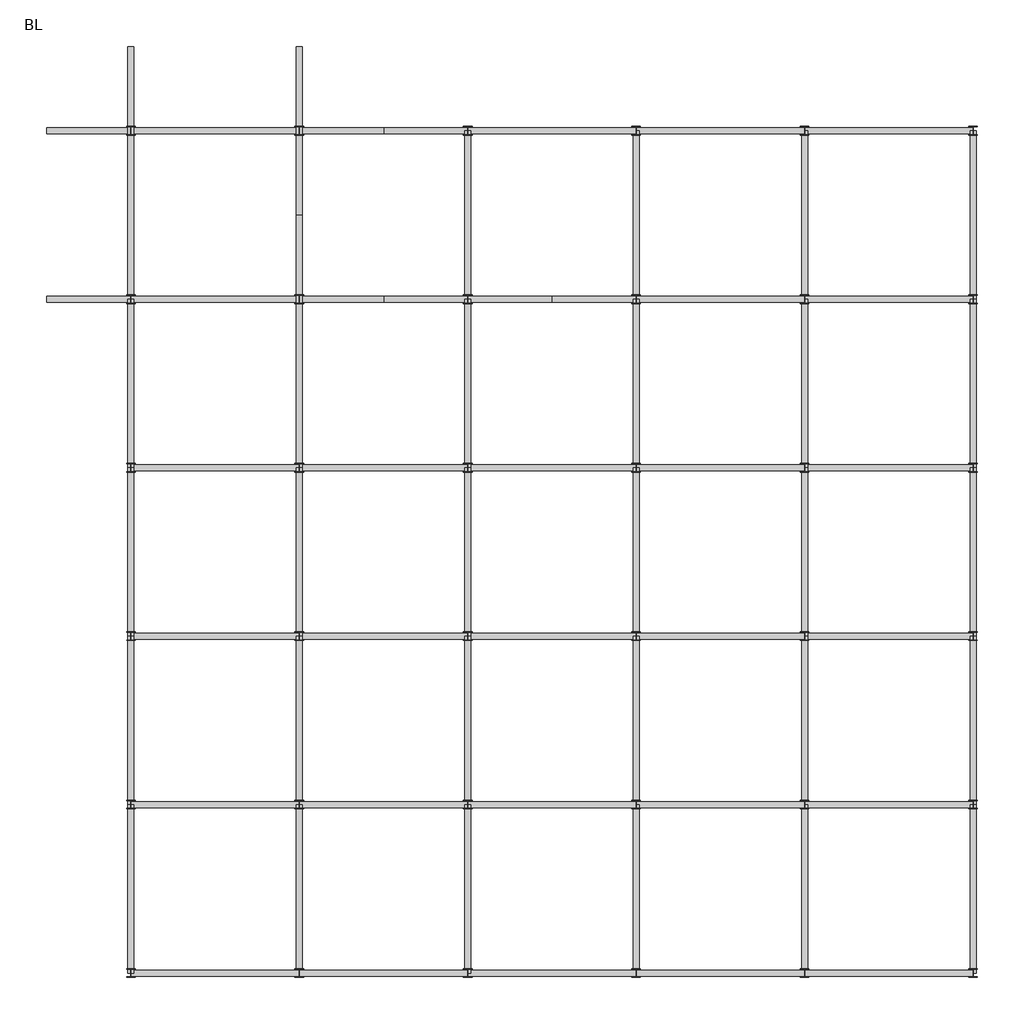
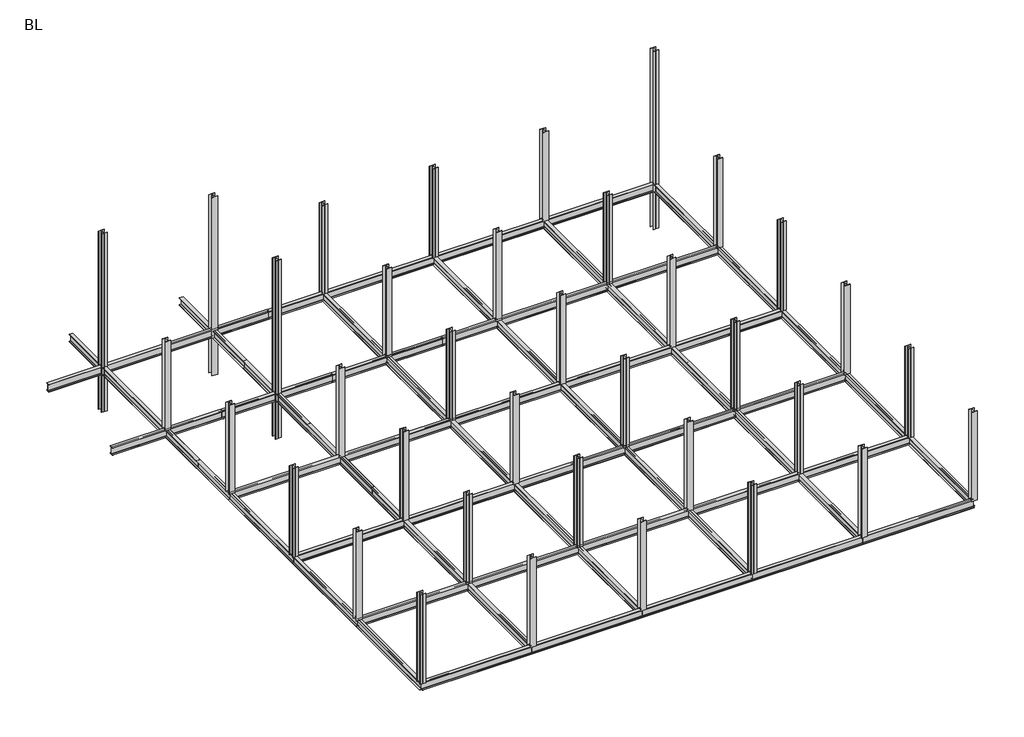
# One storey: 60 beams, 36 columns.
"""IFC4 building model written with IfcOpenShell, lengths in millimetres."""

from ifc_helpers import new_model, si_unit, origin, place, context, project, spatial, transform, mapped, element, save
from components import w_shapes_w14x30_541e514d, w_shapes_w14x30_920474df, w_shapes_column_w10x49_6b2d3d6a, w_shapes_column_w10x49_b9b2aca3

model = new_model("IFC4")

# Units and contexts
model_context = context("Model", 3, world=origin())
ifc_project = project(units=[si_unit("LENGTHUNIT", "METRE", prefix="MILLI")], contexts=[model_context])

# Site, building, storey
site = spatial("IfcSite", under=ifc_project)
building = spatial("IfcBuilding", under=site)
storey = spatial("IfcBuildingStorey", under=building, Name="BL", Elevation=4267.0)

# Beams
placement = place(None, origin())
w_shapes_w14x30_shape = w_shapes_w14x30_541e514d(model_context)
element("IfcBeam", 1, ObjectType="W Shapes : W14X30", at=placement, inside=storey, context=model_context, shape_type="MappedRepresentation", body=[
    mapped(w_shapes_w14x30_shape, transform((-15925.6378857, 14038.8625479, 4091.74), x_axis=(1.0, 0.0, 0.0), y_axis=(0.0, 1.0, 0.0), z_axis=(0.0, 0.0, 1.0))),
])
element("IfcBeam", 2, ObjectType="W Shapes : W14X30", at=placement, inside=storey, context=model_context, shape_type="MappedRepresentation", body=[
    mapped(w_shapes_w14x30_shape, transform((-15925.6378857, 19038.8625479, 4091.74), x_axis=(1.0, 0.0, 0.0), y_axis=(0.0, 1.0, 0.0), z_axis=(0.0, 0.0, 1.0))),
])
element("IfcBeam", 3, ObjectType="W Shapes : W14X30", at=placement, inside=storey, context=model_context, shape_type="MappedRepresentation", body=[
    mapped(w_shapes_w14x30_shape, transform((-13425.6378857, 11538.8625479, 4091.74), x_axis=(0.0, 1.0, 0.0), y_axis=(-1.0, 0.0, 0.0), z_axis=(0.0, 0.0, 1.0))),
])
element("IfcBeam", 4, ObjectType="W Shapes : W14X30", at=placement, inside=storey, context=model_context, shape_type="MappedRepresentation", body=[
    mapped(w_shapes_w14x30_shape, transform((-13425.6378857, 16538.8625479, 4091.74), x_axis=(0.0, 1.0, 0.0), y_axis=(-1.0, 0.0, 0.0), z_axis=(0.0, 0.0, 1.0))),
])
element("IfcBeam", 5, ObjectType="W Shapes : W14X30", at=placement, inside=storey, context=model_context, shape_type="MappedRepresentation", body=[
    mapped(w_shapes_w14x30_shape, transform((-18425.6378857, 16538.8625479, 4091.74), x_axis=(0.0, 1.0, 0.0), y_axis=(-1.0, 0.0, 0.0), z_axis=(0.0, 0.0, 1.0))),
])
element("IfcBeam", 6, ObjectType="W Shapes : W14X30", at=placement, inside=storey, context=model_context, shape_type="MappedRepresentation", body=[
    mapped(w_shapes_w14x30_shape, transform((-10925.6378857, 14038.8625479, 4091.74), x_axis=(1.0, 0.0, 0.0), y_axis=(0.0, 1.0, 0.0), z_axis=(0.0, 0.0, 1.0))),
])
w_shapes_w14x30_2_shape = w_shapes_w14x30_920474df(model_context)
element("IfcBeam", 7, ObjectType="W Shapes : W14X30", at=placement, inside=storey, context=model_context, shape_type="MappedRepresentation", body=[
    mapped(w_shapes_w14x30_2_shape, transform((-15925.6378857, -5961.1374521, 4091.74), x_axis=(1.0, 0.0, 0.0), y_axis=(0.0, 1.0, 0.0), z_axis=(0.0, 0.0, 1.0))),
])
element("IfcBeam", 8, ObjectType="W Shapes : W14X30", at=placement, inside=storey, context=model_context, shape_type="MappedRepresentation", body=[
    mapped(w_shapes_w14x30_2_shape, transform((-10925.6378857, -5961.1374521, 4091.74), x_axis=(1.0, 0.0, 0.0), y_axis=(0.0, 1.0, 0.0), z_axis=(0.0, 0.0, 1.0))),
])
element("IfcBeam", 9, ObjectType="W Shapes : W14X30", at=placement, inside=storey, context=model_context, shape_type="MappedRepresentation", body=[
    mapped(w_shapes_w14x30_2_shape, transform((-5925.6378857, -5961.1374521, 4091.74), x_axis=(1.0, 0.0, 0.0), y_axis=(0.0, 1.0, 0.0), z_axis=(0.0, 0.0, 1.0))),
])
element("IfcBeam", 10, ObjectType="W Shapes : W14X30", at=placement, inside=storey, context=model_context, shape_type="MappedRepresentation", body=[
    mapped(w_shapes_w14x30_2_shape, transform((-925.6378857, -5961.1374521, 4091.74), x_axis=(1.0, 0.0, 0.0), y_axis=(0.0, 1.0, 0.0), z_axis=(0.0, 0.0, 1.0))),
])
element("IfcBeam", 11, ObjectType="W Shapes : W14X30", at=placement, inside=storey, context=model_context, shape_type="MappedRepresentation", body=[
    mapped(w_shapes_w14x30_2_shape, transform((4074.3621143, -5961.1374521, 4091.74), x_axis=(1.0, 0.0, 0.0), y_axis=(0.0, 1.0, 0.0), z_axis=(0.0, 0.0, 1.0))),
])
element("IfcBeam", 12, ObjectType="W Shapes : W14X30", at=placement, inside=storey, context=model_context, shape_type="MappedRepresentation", body=[
    mapped(w_shapes_w14x30_2_shape, transform((-15925.6378857, -961.1374521, 4091.74), x_axis=(1.0, 0.0, 0.0), y_axis=(0.0, 1.0, 0.0), z_axis=(0.0, 0.0, 1.0))),
])
element("IfcBeam", 13, ObjectType="W Shapes : W14X30", at=placement, inside=storey, context=model_context, shape_type="MappedRepresentation", body=[
    mapped(w_shapes_w14x30_2_shape, transform((-10925.6378857, -961.1374521, 4091.74), x_axis=(1.0, 0.0, 0.0), y_axis=(0.0, 1.0, 0.0), z_axis=(0.0, 0.0, 1.0))),
])
element("IfcBeam", 14, ObjectType="W Shapes : W14X30", at=placement, inside=storey, context=model_context, shape_type="MappedRepresentation", body=[
    mapped(w_shapes_w14x30_2_shape, transform((-5925.6378857, -961.1374521, 4091.74), x_axis=(1.0, 0.0, 0.0), y_axis=(0.0, 1.0, 0.0), z_axis=(0.0, 0.0, 1.0))),
])
element("IfcBeam", 15, ObjectType="W Shapes : W14X30", at=placement, inside=storey, context=model_context, shape_type="MappedRepresentation", body=[
    mapped(w_shapes_w14x30_2_shape, transform((-925.6378857, -961.1374521, 4091.74), x_axis=(1.0, 0.0, 0.0), y_axis=(0.0, 1.0, 0.0), z_axis=(0.0, 0.0, 1.0))),
])
element("IfcBeam", 16, ObjectType="W Shapes : W14X30", at=placement, inside=storey, context=model_context, shape_type="MappedRepresentation", body=[
    mapped(w_shapes_w14x30_2_shape, transform((4074.3621143, -961.1374521, 4091.74), x_axis=(1.0, 0.0, 0.0), y_axis=(0.0, 1.0, 0.0), z_axis=(0.0, 0.0, 1.0))),
])
element("IfcBeam", 17, ObjectType="W Shapes : W14X30", at=placement, inside=storey, context=model_context, shape_type="MappedRepresentation", body=[
    mapped(w_shapes_w14x30_2_shape, transform((-15925.6378857, 4038.8625479, 4091.74), x_axis=(1.0, 0.0, 0.0), y_axis=(0.0, 1.0, 0.0), z_axis=(0.0, 0.0, 1.0))),
])
element("IfcBeam", 18, ObjectType="W Shapes : W14X30", at=placement, inside=storey, context=model_context, shape_type="MappedRepresentation", body=[
    mapped(w_shapes_w14x30_2_shape, transform((-10925.6378857, 4038.8625479, 4091.74), x_axis=(1.0, 0.0, 0.0), y_axis=(0.0, 1.0, 0.0), z_axis=(0.0, 0.0, 1.0))),
])
element("IfcBeam", 19, ObjectType="W Shapes : W14X30", at=placement, inside=storey, context=model_context, shape_type="MappedRepresentation", body=[
    mapped(w_shapes_w14x30_2_shape, transform((-5925.6378857, 4038.8625479, 4091.74), x_axis=(1.0, 0.0, 0.0), y_axis=(0.0, 1.0, 0.0), z_axis=(0.0, 0.0, 1.0))),
])
element("IfcBeam", 20, ObjectType="W Shapes : W14X30", at=placement, inside=storey, context=model_context, shape_type="MappedRepresentation", body=[
    mapped(w_shapes_w14x30_2_shape, transform((-925.6378857, 4038.8625479, 4091.74), x_axis=(1.0, 0.0, 0.0), y_axis=(0.0, 1.0, 0.0), z_axis=(0.0, 0.0, 1.0))),
])
element("IfcBeam", 21, ObjectType="W Shapes : W14X30", at=placement, inside=storey, context=model_context, shape_type="MappedRepresentation", body=[
    mapped(w_shapes_w14x30_2_shape, transform((4074.3621143, 4038.8625479, 4091.74), x_axis=(1.0, 0.0, 0.0), y_axis=(0.0, 1.0, 0.0), z_axis=(0.0, 0.0, 1.0))),
])
element("IfcBeam", 22, ObjectType="W Shapes : W14X30", at=placement, inside=storey, context=model_context, shape_type="MappedRepresentation", body=[
    mapped(w_shapes_w14x30_2_shape, transform((-15925.6378857, 9038.8625479, 4091.74), x_axis=(1.0, 0.0, 0.0), y_axis=(0.0, 1.0, 0.0), z_axis=(0.0, 0.0, 1.0))),
])
element("IfcBeam", 23, ObjectType="W Shapes : W14X30", at=placement, inside=storey, context=model_context, shape_type="MappedRepresentation", body=[
    mapped(w_shapes_w14x30_2_shape, transform((-10925.6378857, 9038.8625479, 4091.74), x_axis=(1.0, 0.0, 0.0), y_axis=(0.0, 1.0, 0.0), z_axis=(0.0, 0.0, 1.0))),
])
element("IfcBeam", 24, ObjectType="W Shapes : W14X30", at=placement, inside=storey, context=model_context, shape_type="MappedRepresentation", body=[
    mapped(w_shapes_w14x30_2_shape, transform((-5925.6378857, 9038.8625479, 4091.74), x_axis=(1.0, 0.0, 0.0), y_axis=(0.0, 1.0, 0.0), z_axis=(0.0, 0.0, 1.0))),
])
element("IfcBeam", 25, ObjectType="W Shapes : W14X30", at=placement, inside=storey, context=model_context, shape_type="MappedRepresentation", body=[
    mapped(w_shapes_w14x30_2_shape, transform((-925.6378857, 9038.8625479, 4091.74), x_axis=(1.0, 0.0, 0.0), y_axis=(0.0, 1.0, 0.0), z_axis=(0.0, 0.0, 1.0))),
])
element("IfcBeam", 26, ObjectType="W Shapes : W14X30", at=placement, inside=storey, context=model_context, shape_type="MappedRepresentation", body=[
    mapped(w_shapes_w14x30_2_shape, transform((4074.3621143, 9038.8625479, 4091.74), x_axis=(1.0, 0.0, 0.0), y_axis=(0.0, 1.0, 0.0), z_axis=(0.0, 0.0, 1.0))),
])
element("IfcBeam", 27, ObjectType="W Shapes : W14X30", at=placement, inside=storey, context=model_context, shape_type="MappedRepresentation", body=[
    mapped(w_shapes_w14x30_2_shape, transform((-5925.6378857, 14038.8625479, 4091.74), x_axis=(1.0, 0.0, 0.0), y_axis=(0.0, 1.0, 0.0), z_axis=(0.0, 0.0, 1.0))),
])
element("IfcBeam", 28, ObjectType="W Shapes : W14X30", at=placement, inside=storey, context=model_context, shape_type="MappedRepresentation", body=[
    mapped(w_shapes_w14x30_2_shape, transform((-925.6378857, 14038.8625479, 4091.74), x_axis=(1.0, 0.0, 0.0), y_axis=(0.0, 1.0, 0.0), z_axis=(0.0, 0.0, 1.0))),
])
element("IfcBeam", 29, ObjectType="W Shapes : W14X30", at=placement, inside=storey, context=model_context, shape_type="MappedRepresentation", body=[
    mapped(w_shapes_w14x30_2_shape, transform((4074.3621143, 14038.8625479, 4091.74), x_axis=(1.0, 0.0, 0.0), y_axis=(0.0, 1.0, 0.0), z_axis=(0.0, 0.0, 1.0))),
])
element("IfcBeam", 30, ObjectType="W Shapes : W14X30", at=placement, inside=storey, context=model_context, shape_type="MappedRepresentation", body=[
    mapped(w_shapes_w14x30_2_shape, transform((-10925.6378857, 19038.8625479, 4091.74), x_axis=(1.0, 0.0, 0.0), y_axis=(0.0, 1.0, 0.0), z_axis=(0.0, 0.0, 1.0))),
])
element("IfcBeam", 31, ObjectType="W Shapes : W14X30", at=placement, inside=storey, context=model_context, shape_type="MappedRepresentation", body=[
    mapped(w_shapes_w14x30_2_shape, transform((-5925.6378857, 19038.8625479, 4091.74), x_axis=(1.0, 0.0, 0.0), y_axis=(0.0, 1.0, 0.0), z_axis=(0.0, 0.0, 1.0))),
])
element("IfcBeam", 32, ObjectType="W Shapes : W14X30", at=placement, inside=storey, context=model_context, shape_type="MappedRepresentation", body=[
    mapped(w_shapes_w14x30_2_shape, transform((-925.6378857, 19038.8625479, 4091.74), x_axis=(1.0, 0.0, 0.0), y_axis=(0.0, 1.0, 0.0), z_axis=(0.0, 0.0, 1.0))),
])
element("IfcBeam", 33, ObjectType="W Shapes : W14X30", at=placement, inside=storey, context=model_context, shape_type="MappedRepresentation", body=[
    mapped(w_shapes_w14x30_2_shape, transform((4074.3621143, 19038.8625479, 4091.74), x_axis=(1.0, 0.0, 0.0), y_axis=(0.0, 1.0, 0.0), z_axis=(0.0, 0.0, 1.0))),
])
element("IfcBeam", 34, ObjectType="W Shapes : W14X30", at=placement, inside=storey, context=model_context, shape_type="MappedRepresentation", body=[
    mapped(w_shapes_w14x30_2_shape, transform((6574.3621143, -3461.1374521, 4091.74), x_axis=(0.0, 1.0, 0.0), y_axis=(-1.0, 0.0, 0.0), z_axis=(0.0, 0.0, 1.0))),
])
element("IfcBeam", 35, ObjectType="W Shapes : W14X30", at=placement, inside=storey, context=model_context, shape_type="MappedRepresentation", body=[
    mapped(w_shapes_w14x30_2_shape, transform((6574.3621143, 1538.8625479, 4091.74), x_axis=(0.0, 1.0, 0.0), y_axis=(-1.0, 0.0, 0.0), z_axis=(0.0, 0.0, 1.0))),
])
element("IfcBeam", 36, ObjectType="W Shapes : W14X30", at=placement, inside=storey, context=model_context, shape_type="MappedRepresentation", body=[
    mapped(w_shapes_w14x30_2_shape, transform((6574.3621143, 6538.8625479, 4091.74), x_axis=(0.0, 1.0, 0.0), y_axis=(-1.0, 0.0, 0.0), z_axis=(0.0, 0.0, 1.0))),
])
element("IfcBeam", 37, ObjectType="W Shapes : W14X30", at=placement, inside=storey, context=model_context, shape_type="MappedRepresentation", body=[
    mapped(w_shapes_w14x30_2_shape, transform((6574.3621143, 11538.8625479, 4091.74), x_axis=(0.0, 1.0, 0.0), y_axis=(-1.0, 0.0, 0.0), z_axis=(0.0, 0.0, 1.0))),
])
element("IfcBeam", 38, ObjectType="W Shapes : W14X30", at=placement, inside=storey, context=model_context, shape_type="MappedRepresentation", body=[
    mapped(w_shapes_w14x30_2_shape, transform((6574.3621143, 16538.8625479, 4091.74), x_axis=(0.0, 1.0, 0.0), y_axis=(-1.0, 0.0, 0.0), z_axis=(0.0, 0.0, 1.0))),
])
element("IfcBeam", 39, ObjectType="W Shapes : W14X30", at=placement, inside=storey, context=model_context, shape_type="MappedRepresentation", body=[
    mapped(w_shapes_w14x30_2_shape, transform((1574.3621143, -3461.1374521, 4091.74), x_axis=(0.0, 1.0, 0.0), y_axis=(-1.0, 0.0, 0.0), z_axis=(0.0, 0.0, 1.0))),
])
element("IfcBeam", 40, ObjectType="W Shapes : W14X30", at=placement, inside=storey, context=model_context, shape_type="MappedRepresentation", body=[
    mapped(w_shapes_w14x30_2_shape, transform((1574.3621143, 1538.8625479, 4091.74), x_axis=(0.0, 1.0, 0.0), y_axis=(-1.0, 0.0, 0.0), z_axis=(0.0, 0.0, 1.0))),
])
element("IfcBeam", 41, ObjectType="W Shapes : W14X30", at=placement, inside=storey, context=model_context, shape_type="MappedRepresentation", body=[
    mapped(w_shapes_w14x30_2_shape, transform((1574.3621143, 6538.8625479, 4091.74), x_axis=(0.0, 1.0, 0.0), y_axis=(-1.0, 0.0, 0.0), z_axis=(0.0, 0.0, 1.0))),
])
element("IfcBeam", 42, ObjectType="W Shapes : W14X30", at=placement, inside=storey, context=model_context, shape_type="MappedRepresentation", body=[
    mapped(w_shapes_w14x30_2_shape, transform((1574.3621143, 11538.8625479, 4091.74), x_axis=(0.0, 1.0, 0.0), y_axis=(-1.0, 0.0, 0.0), z_axis=(0.0, 0.0, 1.0))),
])
element("IfcBeam", 43, ObjectType="W Shapes : W14X30", at=placement, inside=storey, context=model_context, shape_type="MappedRepresentation", body=[
    mapped(w_shapes_w14x30_2_shape, transform((1574.3621143, 16538.8625479, 4091.74), x_axis=(0.0, 1.0, 0.0), y_axis=(-1.0, 0.0, 0.0), z_axis=(0.0, 0.0, 1.0))),
])
element("IfcBeam", 44, ObjectType="W Shapes : W14X30", at=placement, inside=storey, context=model_context, shape_type="MappedRepresentation", body=[
    mapped(w_shapes_w14x30_2_shape, transform((-3425.6378857, -3461.1374521, 4091.74), x_axis=(0.0, 1.0, 0.0), y_axis=(-1.0, 0.0, 0.0), z_axis=(0.0, 0.0, 1.0))),
])
element("IfcBeam", 45, ObjectType="W Shapes : W14X30", at=placement, inside=storey, context=model_context, shape_type="MappedRepresentation", body=[
    mapped(w_shapes_w14x30_2_shape, transform((-3425.6378857, 1538.8625479, 4091.74), x_axis=(0.0, 1.0, 0.0), y_axis=(-1.0, 0.0, 0.0), z_axis=(0.0, 0.0, 1.0))),
])
element("IfcBeam", 46, ObjectType="W Shapes : W14X30", at=placement, inside=storey, context=model_context, shape_type="MappedRepresentation", body=[
    mapped(w_shapes_w14x30_2_shape, transform((-3425.6378857, 6538.8625479, 4091.74), x_axis=(0.0, 1.0, 0.0), y_axis=(-1.0, 0.0, 0.0), z_axis=(0.0, 0.0, 1.0))),
])
element("IfcBeam", 47, ObjectType="W Shapes : W14X30", at=placement, inside=storey, context=model_context, shape_type="MappedRepresentation", body=[
    mapped(w_shapes_w14x30_2_shape, transform((-3425.6378857, 11538.8625479, 4091.74), x_axis=(0.0, 1.0, 0.0), y_axis=(-1.0, 0.0, 0.0), z_axis=(0.0, 0.0, 1.0))),
])
element("IfcBeam", 48, ObjectType="W Shapes : W14X30", at=placement, inside=storey, context=model_context, shape_type="MappedRepresentation", body=[
    mapped(w_shapes_w14x30_2_shape, transform((-3425.6378857, 16538.8625479, 4091.74), x_axis=(0.0, 1.0, 0.0), y_axis=(-1.0, 0.0, 0.0), z_axis=(0.0, 0.0, 1.0))),
])
element("IfcBeam", 49, ObjectType="W Shapes : W14X30", at=placement, inside=storey, context=model_context, shape_type="MappedRepresentation", body=[
    mapped(w_shapes_w14x30_2_shape, transform((-8425.6378857, -3461.1374521, 4091.74), x_axis=(0.0, 1.0, 0.0), y_axis=(-1.0, 0.0, 0.0), z_axis=(0.0, 0.0, 1.0))),
])
element("IfcBeam", 50, ObjectType="W Shapes : W14X30", at=placement, inside=storey, context=model_context, shape_type="MappedRepresentation", body=[
    mapped(w_shapes_w14x30_2_shape, transform((-8425.6378857, 1538.8625479, 4091.74), x_axis=(0.0, 1.0, 0.0), y_axis=(-1.0, 0.0, 0.0), z_axis=(0.0, 0.0, 1.0))),
])
element("IfcBeam", 51, ObjectType="W Shapes : W14X30", at=placement, inside=storey, context=model_context, shape_type="MappedRepresentation", body=[
    mapped(w_shapes_w14x30_2_shape, transform((-8425.6378857, 6538.8625479, 4091.74), x_axis=(0.0, 1.0, 0.0), y_axis=(-1.0, 0.0, 0.0), z_axis=(0.0, 0.0, 1.0))),
])
element("IfcBeam", 52, ObjectType="W Shapes : W14X30", at=placement, inside=storey, context=model_context, shape_type="MappedRepresentation", body=[
    mapped(w_shapes_w14x30_2_shape, transform((-8425.6378857, 11538.8625479, 4091.74), x_axis=(0.0, 1.0, 0.0), y_axis=(-1.0, 0.0, 0.0), z_axis=(0.0, 0.0, 1.0))),
])
element("IfcBeam", 53, ObjectType="W Shapes : W14X30", at=placement, inside=storey, context=model_context, shape_type="MappedRepresentation", body=[
    mapped(w_shapes_w14x30_2_shape, transform((-8425.6378857, 16538.8625479, 4091.74), x_axis=(0.0, 1.0, 0.0), y_axis=(-1.0, 0.0, 0.0), z_axis=(0.0, 0.0, 1.0))),
])
element("IfcBeam", 54, ObjectType="W Shapes : W14X30", at=placement, inside=storey, context=model_context, shape_type="MappedRepresentation", body=[
    mapped(w_shapes_w14x30_2_shape, transform((-13425.6378857, -3461.1374521, 4091.74), x_axis=(0.0, 1.0, 0.0), y_axis=(-1.0, 0.0, 0.0), z_axis=(0.0, 0.0, 1.0))),
])
element("IfcBeam", 55, ObjectType="W Shapes : W14X30", at=placement, inside=storey, context=model_context, shape_type="MappedRepresentation", body=[
    mapped(w_shapes_w14x30_2_shape, transform((-13425.6378857, 1538.8625479, 4091.74), x_axis=(0.0, 1.0, 0.0), y_axis=(-1.0, 0.0, 0.0), z_axis=(0.0, 0.0, 1.0))),
])
element("IfcBeam", 56, ObjectType="W Shapes : W14X30", at=placement, inside=storey, context=model_context, shape_type="MappedRepresentation", body=[
    mapped(w_shapes_w14x30_2_shape, transform((-13425.6378857, 6538.8625479, 4091.74), x_axis=(0.0, 1.0, 0.0), y_axis=(-1.0, 0.0, 0.0), z_axis=(0.0, 0.0, 1.0))),
])
element("IfcBeam", 57, ObjectType="W Shapes : W14X30", at=placement, inside=storey, context=model_context, shape_type="MappedRepresentation", body=[
    mapped(w_shapes_w14x30_2_shape, transform((-18425.6378857, -3461.1374521, 4091.74), x_axis=(0.0, 1.0, 0.0), y_axis=(-1.0, 0.0, 0.0), z_axis=(0.0, 0.0, 1.0))),
])
element("IfcBeam", 58, ObjectType="W Shapes : W14X30", at=placement, inside=storey, context=model_context, shape_type="MappedRepresentation", body=[
    mapped(w_shapes_w14x30_2_shape, transform((-18425.6378857, 1538.8625479, 4091.74), x_axis=(0.0, 1.0, 0.0), y_axis=(-1.0, 0.0, 0.0), z_axis=(0.0, 0.0, 1.0))),
])
element("IfcBeam", 59, ObjectType="W Shapes : W14X30", at=placement, inside=storey, context=model_context, shape_type="MappedRepresentation", body=[
    mapped(w_shapes_w14x30_2_shape, transform((-18425.6378857, 6538.8625479, 4091.74), x_axis=(0.0, 1.0, 0.0), y_axis=(-1.0, 0.0, 0.0), z_axis=(0.0, 0.0, 1.0))),
])
element("IfcBeam", 60, ObjectType="W Shapes : W14X30", at=placement, inside=storey, context=model_context, shape_type="MappedRepresentation", body=[
    mapped(w_shapes_w14x30_2_shape, transform((-18425.6378857, 11538.8625479, 4091.74), x_axis=(0.0, 1.0, 0.0), y_axis=(-1.0, 0.0, 0.0), z_axis=(0.0, 0.0, 1.0))),
])

# Columns
w_shapes_column_w10x49_shape = w_shapes_column_w10x49_6b2d3d6a(model_context)
element("IfcColumn", 61, ObjectType="W Shapes-Column : W10X49", at=placement, inside=storey, context=model_context, shape_type="MappedRepresentation", body=[
    mapped(w_shapes_column_w10x49_shape, transform((6574.3621143, -5961.1374521, 0.0), x_axis=(1.0, 0.0, 0.0), y_axis=(0.0, 1.0, 0.0), z_axis=(0.0, 0.0, 1.0))),
])
element("IfcColumn", 62, ObjectType="W Shapes-Column : W10X49", at=placement, inside=storey, context=model_context, shape_type="MappedRepresentation", body=[
    mapped(w_shapes_column_w10x49_shape, transform((1574.3621143, -5961.1374521, 0.0), x_axis=(1.0, 0.0, 0.0), y_axis=(0.0, 1.0, 0.0), z_axis=(0.0, 0.0, 1.0))),
])
element("IfcColumn", 63, ObjectType="W Shapes-Column : W10X49", at=placement, inside=storey, context=model_context, shape_type="MappedRepresentation", body=[
    mapped(w_shapes_column_w10x49_shape, transform((-3425.6378857, -5961.1374521, 0.0), x_axis=(1.0, 0.0, 0.0), y_axis=(0.0, 1.0, 0.0), z_axis=(0.0, 0.0, 1.0))),
])
element("IfcColumn", 64, ObjectType="W Shapes-Column : W10X49", at=placement, inside=storey, context=model_context, shape_type="MappedRepresentation", body=[
    mapped(w_shapes_column_w10x49_shape, transform((-8425.6378857, -5961.1374521, 0.0), x_axis=(1.0, 0.0, 0.0), y_axis=(0.0, 1.0, 0.0), z_axis=(0.0, 0.0, 1.0))),
])
element("IfcColumn", 65, ObjectType="W Shapes-Column : W10X49", at=placement, inside=storey, context=model_context, shape_type="MappedRepresentation", body=[
    mapped(w_shapes_column_w10x49_shape, transform((-13425.6378857, -5961.1374521, 0.0), x_axis=(1.0, 0.0, 0.0), y_axis=(0.0, 1.0, 0.0), z_axis=(0.0, 0.0, 1.0))),
])
element("IfcColumn", 66, ObjectType="W Shapes-Column : W10X49", at=placement, inside=storey, context=model_context, shape_type="MappedRepresentation", body=[
    mapped(w_shapes_column_w10x49_shape, transform((-18425.6378857, -5961.1374521, 0.0), x_axis=(1.0, 0.0, 0.0), y_axis=(0.0, 1.0, 0.0), z_axis=(0.0, 0.0, 1.0))),
])
element("IfcColumn", 67, ObjectType="W Shapes-Column : W10X49", at=placement, inside=storey, context=model_context, shape_type="MappedRepresentation", body=[
    mapped(w_shapes_column_w10x49_shape, transform((6574.3621143, -961.1374521, 0.0), x_axis=(1.0, 0.0, 0.0), y_axis=(0.0, 1.0, 0.0), z_axis=(0.0, 0.0, 1.0))),
])
element("IfcColumn", 68, ObjectType="W Shapes-Column : W10X49", at=placement, inside=storey, context=model_context, shape_type="MappedRepresentation", body=[
    mapped(w_shapes_column_w10x49_shape, transform((1574.3621143, -961.1374521, 0.0), x_axis=(1.0, 0.0, 0.0), y_axis=(0.0, 1.0, 0.0), z_axis=(0.0, 0.0, 1.0))),
])
element("IfcColumn", 69, ObjectType="W Shapes-Column : W10X49", at=placement, inside=storey, context=model_context, shape_type="MappedRepresentation", body=[
    mapped(w_shapes_column_w10x49_shape, transform((-3425.6378857, -961.1374521, 0.0), x_axis=(1.0, 0.0, 0.0), y_axis=(0.0, 1.0, 0.0), z_axis=(0.0, 0.0, 1.0))),
])
element("IfcColumn", 70, ObjectType="W Shapes-Column : W10X49", at=placement, inside=storey, context=model_context, shape_type="MappedRepresentation", body=[
    mapped(w_shapes_column_w10x49_shape, transform((-8425.6378857, -961.1374521, 0.0), x_axis=(1.0, 0.0, 0.0), y_axis=(0.0, 1.0, 0.0), z_axis=(0.0, 0.0, 1.0))),
])
element("IfcColumn", 71, ObjectType="W Shapes-Column : W10X49", at=placement, inside=storey, context=model_context, shape_type="MappedRepresentation", body=[
    mapped(w_shapes_column_w10x49_shape, transform((-13425.6378857, -961.1374521, 0.0), x_axis=(1.0, 0.0, 0.0), y_axis=(0.0, 1.0, 0.0), z_axis=(0.0, 0.0, 1.0))),
])
element("IfcColumn", 72, ObjectType="W Shapes-Column : W10X49", at=placement, inside=storey, context=model_context, shape_type="MappedRepresentation", body=[
    mapped(w_shapes_column_w10x49_shape, transform((-18425.6378857, -961.1374521, 0.0), x_axis=(1.0, 0.0, 0.0), y_axis=(0.0, 1.0, 0.0), z_axis=(0.0, 0.0, 1.0))),
])
element("IfcColumn", 73, ObjectType="W Shapes-Column : W10X49", at=placement, inside=storey, context=model_context, shape_type="MappedRepresentation", body=[
    mapped(w_shapes_column_w10x49_shape, transform((6574.3621143, 4038.8625479, 0.0), x_axis=(1.0, 0.0, 0.0), y_axis=(0.0, 1.0, 0.0), z_axis=(0.0, 0.0, 1.0))),
])
element("IfcColumn", 74, ObjectType="W Shapes-Column : W10X49", at=placement, inside=storey, context=model_context, shape_type="MappedRepresentation", body=[
    mapped(w_shapes_column_w10x49_shape, transform((1574.3621143, 4038.8625479, 0.0), x_axis=(1.0, 0.0, 0.0), y_axis=(0.0, 1.0, 0.0), z_axis=(0.0, 0.0, 1.0))),
])
element("IfcColumn", 75, ObjectType="W Shapes-Column : W10X49", at=placement, inside=storey, context=model_context, shape_type="MappedRepresentation", body=[
    mapped(w_shapes_column_w10x49_shape, transform((-3425.6378857, 4038.8625479, 0.0), x_axis=(1.0, 0.0, 0.0), y_axis=(0.0, 1.0, 0.0), z_axis=(0.0, 0.0, 1.0))),
])
element("IfcColumn", 76, ObjectType="W Shapes-Column : W10X49", at=placement, inside=storey, context=model_context, shape_type="MappedRepresentation", body=[
    mapped(w_shapes_column_w10x49_shape, transform((-8425.6378857, 4038.8625479, 0.0), x_axis=(1.0, 0.0, 0.0), y_axis=(0.0, 1.0, 0.0), z_axis=(0.0, 0.0, 1.0))),
])
element("IfcColumn", 77, ObjectType="W Shapes-Column : W10X49", at=placement, inside=storey, context=model_context, shape_type="MappedRepresentation", body=[
    mapped(w_shapes_column_w10x49_shape, transform((-13425.6378857, 4038.8625479, 0.0), x_axis=(1.0, 0.0, 0.0), y_axis=(0.0, 1.0, 0.0), z_axis=(0.0, 0.0, 1.0))),
])
element("IfcColumn", 78, ObjectType="W Shapes-Column : W10X49", at=placement, inside=storey, context=model_context, shape_type="MappedRepresentation", body=[
    mapped(w_shapes_column_w10x49_shape, transform((-18425.6378857, 4038.8625479, 0.0), x_axis=(1.0, 0.0, 0.0), y_axis=(0.0, 1.0, 0.0), z_axis=(0.0, 0.0, 1.0))),
])
element("IfcColumn", 79, ObjectType="W Shapes-Column : W10X49", at=placement, inside=storey, context=model_context, shape_type="MappedRepresentation", body=[
    mapped(w_shapes_column_w10x49_shape, transform((6574.3621143, 9038.8625479, 0.0), x_axis=(1.0, 0.0, 0.0), y_axis=(0.0, 1.0, 0.0), z_axis=(0.0, 0.0, 1.0))),
])
element("IfcColumn", 80, ObjectType="W Shapes-Column : W10X49", at=placement, inside=storey, context=model_context, shape_type="MappedRepresentation", body=[
    mapped(w_shapes_column_w10x49_shape, transform((1574.3621143, 9038.8625479, 0.0), x_axis=(1.0, 0.0, 0.0), y_axis=(0.0, 1.0, 0.0), z_axis=(0.0, 0.0, 1.0))),
])
element("IfcColumn", 81, ObjectType="W Shapes-Column : W10X49", at=placement, inside=storey, context=model_context, shape_type="MappedRepresentation", body=[
    mapped(w_shapes_column_w10x49_shape, transform((-3425.6378857, 9038.8625479, 0.0), x_axis=(1.0, 0.0, 0.0), y_axis=(0.0, 1.0, 0.0), z_axis=(0.0, 0.0, 1.0))),
])
element("IfcColumn", 82, ObjectType="W Shapes-Column : W10X49", at=placement, inside=storey, context=model_context, shape_type="MappedRepresentation", body=[
    mapped(w_shapes_column_w10x49_shape, transform((-8425.6378857, 9038.8625479, 0.0), x_axis=(1.0, 0.0, 0.0), y_axis=(0.0, 1.0, 0.0), z_axis=(0.0, 0.0, 1.0))),
])
element("IfcColumn", 83, ObjectType="W Shapes-Column : W10X49", at=placement, inside=storey, context=model_context, shape_type="MappedRepresentation", body=[
    mapped(w_shapes_column_w10x49_shape, transform((-13425.6378857, 9038.8625479, 0.0), x_axis=(1.0, 0.0, 0.0), y_axis=(0.0, 1.0, 0.0), z_axis=(0.0, 0.0, 1.0))),
])
element("IfcColumn", 84, ObjectType="W Shapes-Column : W10X49", at=placement, inside=storey, context=model_context, shape_type="MappedRepresentation", body=[
    mapped(w_shapes_column_w10x49_shape, transform((-18425.6378857, 9038.8625479, 0.0), x_axis=(1.0, 0.0, 0.0), y_axis=(0.0, 1.0, 0.0), z_axis=(0.0, 0.0, 1.0))),
])
element("IfcColumn", 85, ObjectType="W Shapes-Column : W10X49", at=placement, inside=storey, context=model_context, shape_type="MappedRepresentation", body=[
    mapped(w_shapes_column_w10x49_shape, transform((6574.3621143, 14038.8625479, 0.0), x_axis=(1.0, 0.0, 0.0), y_axis=(0.0, 1.0, 0.0), z_axis=(0.0, 0.0, 1.0))),
])
element("IfcColumn", 86, ObjectType="W Shapes-Column : W10X49", at=placement, inside=storey, context=model_context, shape_type="MappedRepresentation", body=[
    mapped(w_shapes_column_w10x49_shape, transform((1574.3621143, 14038.8625479, 0.0), x_axis=(1.0, 0.0, 0.0), y_axis=(0.0, 1.0, 0.0), z_axis=(0.0, 0.0, 1.0))),
])
element("IfcColumn", 87, ObjectType="W Shapes-Column : W10X49", at=placement, inside=storey, context=model_context, shape_type="MappedRepresentation", body=[
    mapped(w_shapes_column_w10x49_shape, transform((-3425.6378857, 14038.8625479, 0.0), x_axis=(1.0, 0.0, 0.0), y_axis=(0.0, 1.0, 0.0), z_axis=(0.0, 0.0, 1.0))),
])
element("IfcColumn", 88, ObjectType="W Shapes-Column : W10X49", at=placement, inside=storey, context=model_context, shape_type="MappedRepresentation", body=[
    mapped(w_shapes_column_w10x49_shape, transform((-8425.6378857, 14038.8625479, 0.0), x_axis=(1.0, 0.0, 0.0), y_axis=(0.0, 1.0, 0.0), z_axis=(0.0, 0.0, 1.0))),
])
element("IfcColumn", 89, ObjectType="W Shapes-Column : W10X49", at=placement, inside=storey, context=model_context, shape_type="MappedRepresentation", body=[
    mapped(w_shapes_column_w10x49_shape, transform((-18425.6378857, 14038.8625479, 0.0), x_axis=(1.0, 0.0, 0.0), y_axis=(0.0, 1.0, 0.0), z_axis=(0.0, 0.0, 1.0))),
])
element("IfcColumn", 90, ObjectType="W Shapes-Column : W10X49", at=placement, inside=storey, context=model_context, shape_type="MappedRepresentation", body=[
    mapped(w_shapes_column_w10x49_shape, transform((1574.3621143, 19038.8625479, 0.0), x_axis=(1.0, 0.0, 0.0), y_axis=(0.0, 1.0, 0.0), z_axis=(0.0, 0.0, 1.0))),
])
element("IfcColumn", 91, ObjectType="W Shapes-Column : W10X49", at=placement, inside=storey, context=model_context, shape_type="MappedRepresentation", body=[
    mapped(w_shapes_column_w10x49_shape, transform((-3425.6378857, 19038.8625479, 0.0), x_axis=(1.0, 0.0, 0.0), y_axis=(0.0, 1.0, 0.0), z_axis=(0.0, 0.0, 1.0))),
])
element("IfcColumn", 92, ObjectType="W Shapes-Column : W10X49", at=placement, inside=storey, context=model_context, shape_type="MappedRepresentation", body=[
    mapped(w_shapes_column_w10x49_shape, transform((-8425.6378857, 19038.8625479, 0.0), x_axis=(1.0, 0.0, 0.0), y_axis=(0.0, 1.0, 0.0), z_axis=(0.0, 0.0, 1.0))),
])
w_shapes_column_w10x49_2_shape = w_shapes_column_w10x49_b9b2aca3(model_context)
element("IfcColumn", 93, ObjectType="W Shapes-Column : W10X49", at=placement, inside=storey, context=model_context, shape_type="MappedRepresentation", body=[
    mapped(w_shapes_column_w10x49_2_shape, transform((-13425.6378857, 14038.8625479, 0.0), x_axis=(1.0, 0.0, 0.0), y_axis=(0.0, 1.0, 0.0), z_axis=(0.0, 0.0, 1.0))),
])
element("IfcColumn", 94, ObjectType="W Shapes-Column : W10X49", at=placement, inside=storey, context=model_context, shape_type="MappedRepresentation", body=[
    mapped(w_shapes_column_w10x49_2_shape, transform((6574.3621143, 19038.8625479, 0.0), x_axis=(1.0, 0.0, 0.0), y_axis=(0.0, 1.0, 0.0), z_axis=(0.0, 0.0, 1.0))),
])
element("IfcColumn", 95, ObjectType="W Shapes-Column : W10X49", at=placement, inside=storey, context=model_context, shape_type="MappedRepresentation", body=[
    mapped(w_shapes_column_w10x49_2_shape, transform((-13425.6378857, 19038.8625479, 0.0), x_axis=(1.0, 0.0, 0.0), y_axis=(0.0, 1.0, 0.0), z_axis=(0.0, 0.0, 1.0))),
])
element("IfcColumn", 96, ObjectType="W Shapes-Column : W10X49", at=placement, inside=storey, context=model_context, shape_type="MappedRepresentation", body=[
    mapped(w_shapes_column_w10x49_2_shape, transform((-18425.6378857, 19038.8625479, 0.0), x_axis=(1.0, 0.0, 0.0), y_axis=(0.0, 1.0, 0.0), z_axis=(0.0, 0.0, 1.0))),
])

save(model, "model.ifc")

# Revit data of these elements
# Type "W Shapes : W14X30"
#   Section Name Key = "W14X30"
#   Width = 6.730"
#   Web Thickness = 0.270"
#   Web Fillet = 0.400"
#   Warping Constant = 887.00 in⁶
#   Torsional Moment of Inertia = 0.38 in⁴
#   Section Area = 8.85 in²
#   Plastic Modulus weak axis = 8.99 in³
#   Plastic Modulus strong axis = 47.30 in³
#   Perimeter = 4.441 ft²/ft
#   Nominal Weight = 30.00 lbf/ft
#   Moment of Inertia weak axis = 19.60 in⁴
#   Moment of Inertia strong axis = 291.00 in⁴
#   Height = 13.800"
#   Flange Thickness = 0.385"
#   Elastic Modulus weak axis = 5.82 in³
#   Elastic Modulus strong axis = 42.00 in³
#   Clear Web Height = 0' - 11 5/8"
#   Centroid Vertical = 6.900"
#   Centroid Horizontal = 3.365"
#   Bolt Spacing = 0' - 3 1/2"
#   Length [instance default] = 1524 mm
#   Structural Material [instance default] = Steel ASTM A992
#   Principal Axes Angle = 0
# Type "W Shapes-Column : W10X49"
#   Section Name Key = "W10X49"
#   Width = 10.000"
#   Web Thickness = 0.340"
#   Web Fillet = 0.500"
#   Warping Constant = 2070.00 in⁶
#   Torsional Moment of Inertia = 1.39 in⁴
#   Section Area = 14.40 in²
#   Plastic Modulus weak axis = 28.30 in³
#   Plastic Modulus strong axis = 60.40 in³
#   Perimeter = 4.875 ft²/ft
#   Nominal Weight = 49.00 lbf/ft
#   Moment of Inertia weak axis = 93.40 in⁴
#   Moment of Inertia strong axis = 272.00 in⁴
#   Height = 10.000"
#   Flange Thickness = 0.560"
#   Elastic Modulus weak axis = 18.70 in³
#   Elastic Modulus strong axis = 54.60 in³
#   Clear Web Height = 0' - 7 1/2"
#   Centroid Vertical = 5.000"
#   Centroid Horizontal = 5.000"
#   Bolt Spacing = 0' - 5 1/2"
#   Structural Material [instance default] = Steel ASTM A992
#   Principal Axes Angle = 0
# Elements 1, 2, 3, 4, 5, 6, 7, 8, 9, 10, 11, 12, 13, 14, 15, 16, 17, 18, 19, 20, 21, 22, 23, 24, 25, 26, 27, 28, 29, 30, 31, 32, 33, 34, 35, 36, 37, 38, 39, 40, 41, 42, 43, 44, 45, 46, 47, 48, 49, 50, 51, 52, 53, 54, 55, 56, 57, 58, 59, 60 (IfcBeam, "W Shapes : W14X30")
#   Length = 5000 mm
#   Structural Material = Steel ASTM A992
#   Phase Created = New Construction
#   Materials on its faces: "Steel ASTM A992"
# Elements 61, 62, 63, 64, 65, 66, 67, 68, 69, 70, 71, 72, 73, 74, 75, 76, 77, 78, 79, 80, 81, 82, 83, 84, 85, 86, 87, 88, 89, 90, 91, 92, 93, 94, 95, 96 (IfcColumn, "W Shapes-Column : W10X49")
#   Structural Material = Steel ASTM A992
#   Phase Created = New Construction
#   Materials on its faces: "Steel ASTM A992"
# Materials
#   "Steel ASTM A992": class "Metal", colour RGB 199 199 199, transparency 0, Description = "Structural steel 50ksi", Cost = 0
